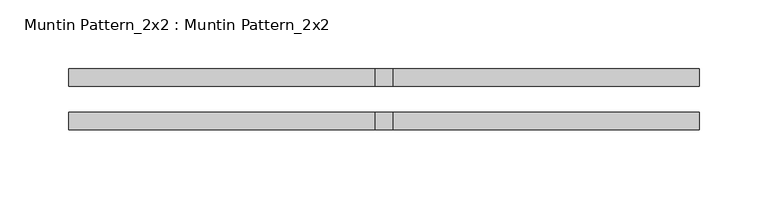
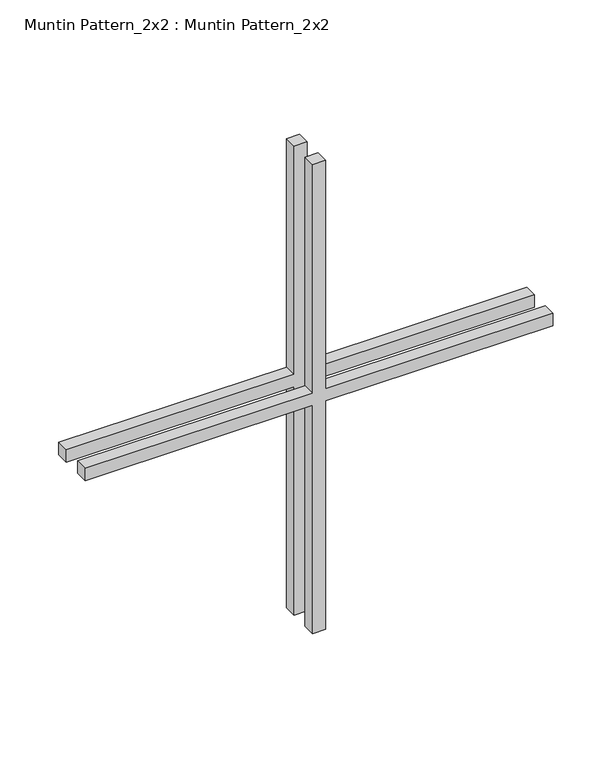
"""IFC4 building model written with IfcOpenShell, lengths in millimetres: proxy geometry, Muntin Pattern_2x2 : Muntin Pattern_2x2."""

from ifc_helpers import new_model, si_unit, frame, origin, place, context, project, spatial, polyline, outline, extrude, source, transform, mapped, element, save


def muntin_pattern_2x2_muntin_pattern_2x2_3e1923be(model_context):
    return source(origin(), model_context, "Body", "SweptSolid", [
        extrude(outline(polyline([(249.2375, -6.35), (249.2375, -229.39375), (236.5375, -229.39375), (236.5375, -6.35), (0.0, -6.35), (0.0, 6.35), (236.5375, 6.35), (236.5375, 229.39375), (249.2375, 229.39375), (249.2375, 6.35), (485.775, 6.35), (485.775, -6.35), (249.2375, -6.35)])), frame((0.0, 9.525, 0.0), z_axis=(0.0, 1.0, 0.0), x_axis=(0.0, 0.0, 1.0)), (0.0, 0.0, 1.0), 12.7),
        extrude(outline(polyline([(249.2375, -6.35), (249.2375, -229.39375), (236.5375, -229.39375), (236.5375, -6.35), (0.0, -6.35), (0.0, 6.35), (236.5375, 6.35), (236.5375, 229.39375), (249.2375, 229.39375), (249.2375, 6.35), (485.775, 6.35), (485.775, -6.35), (249.2375, -6.35)])), frame((0.0, -22.225, 0.0), z_axis=(0.0, 1.0, 0.0), x_axis=(0.0, 0.0, 1.0)), (0.0, 0.0, 1.0), 12.7),
    ])


if __name__ == "__main__":
    model = new_model("IFC4")
    model_context = context("Model", 3, world=origin())
    ifc_project = project(units=[si_unit("LENGTHUNIT", "METRE", prefix="MILLI")], contexts=[model_context])
    site = spatial("IfcSite", under=ifc_project)
    building = spatial("IfcBuilding", under=site)
    placement = place(None, origin())
    muntin_pattern_2x2_muntin_pattern_2x2_shape = muntin_pattern_2x2_muntin_pattern_2x2_3e1923be(model_context)
    element("IfcBuildingElementProxy", 1, Name="Muntin Pattern_2x2 : Muntin Pattern_2x2", ObjectType="Muntin Pattern_2x2 : Muntin Pattern_2x2", at=placement, inside=building, context=model_context, shape_type="MappedRepresentation", body=[
        mapped(muntin_pattern_2x2_muntin_pattern_2x2_shape, transform((0.0, 0.0, 0.0), x_axis=(1.0, 0.0, 0.0), y_axis=(0.0, 1.0, 0.0), z_axis=(0.0, 0.0, 1.0))),
    ])
    save(model, "model.ifc")

# Revit data of these elements
# Type "Muntin Pattern_2x2 : Muntin Pattern_2x2"
#   Width [instance default] = 4' - 0"
#   Thickness = 0' - 0 1/2"
#   Height [instance default] = 4' - 0"
#   Distance = 0' - 0 3/4"
#   Interior Material [instance default] = none
#   Exterior Material [instance default] = none
#   Default Elevation = 0
# Element 1 (IfcBuildingElementProxy, "Muntin Pattern_2x2 : Muntin Pattern_2x2")
#   Width = 1' - 6 1/16"
#   Height = 1' - 7 1/8"
#   Interior Material = Wood - Stained
#   Exterior Material = Clad - White
#   Materials on its faces: "Clad - White", "Wood - Stained"
# Materials
#   "Clad - White": class "Wood", colour RGB 242 242 238, transparency 0, Cost = 0
#   "Wood - Stained": class "Wood", colour RGB 224 178 126, transparency 0, Cost = 0
